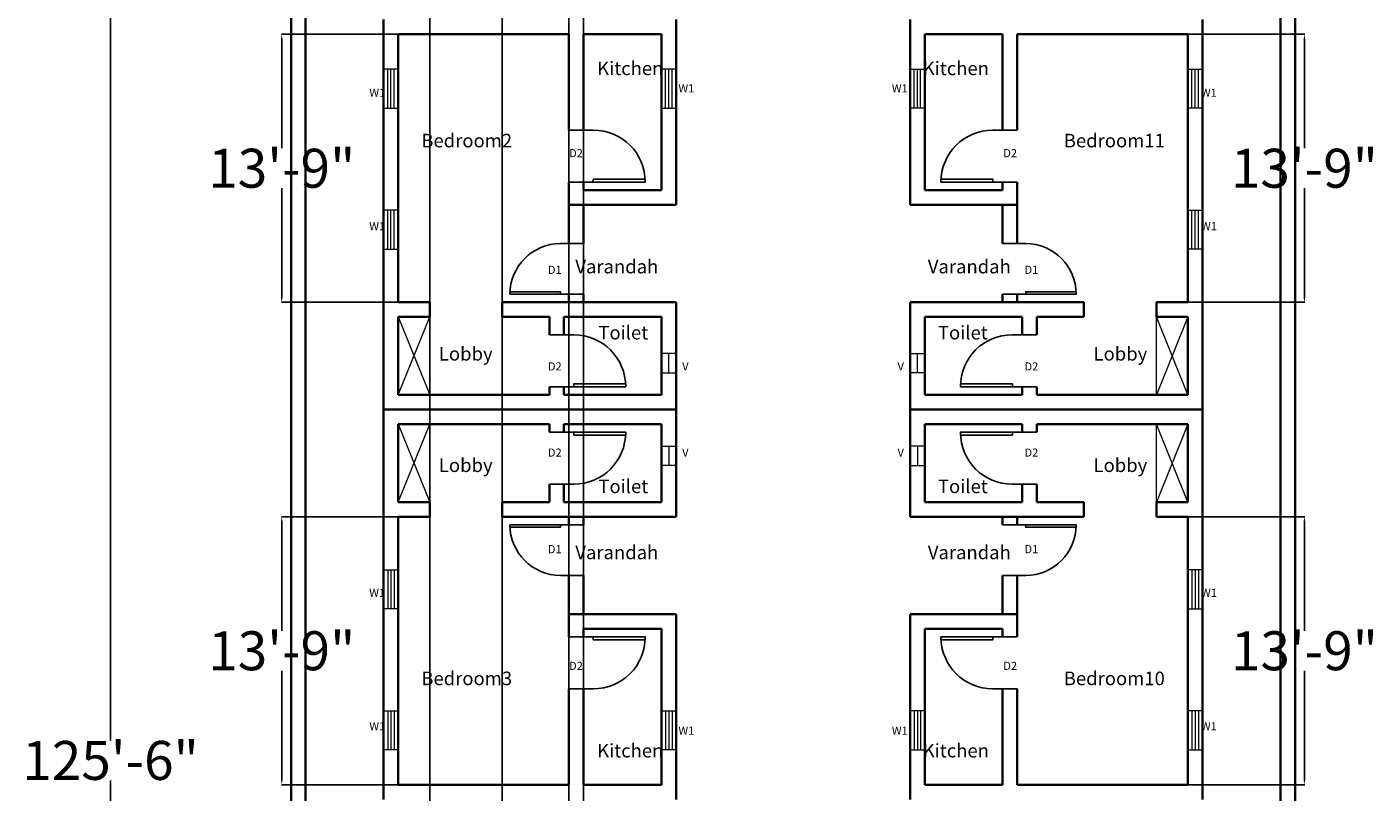
# Model space of a CAD drawing. Units: inches. Extents: x -205 to 674, y 63 to 1798.
# Tile 2 of 4: x -205 to 624, y 888 to 1359. Entities that reach past the tile are written whole.
import ezdxf

# ---------------------------------------------------------------- set-up
doc = ezdxf.new("R2010")
doc.units = ezdxf.units.IN
doc.header["$MEASUREMENT"] = 0
doc.layers.get('0').update_dxf_attribs({"color": 70})
for name, color, linetype, lineweight in [('A-ANNO-DIMS', 240, 'Continuous', 18), ('A-ANNO-TEXT', 240, 'Continuous', 18), ('A-AREA-IDEN', 240, 'Continuous', 18), ('A-WALL', 70, 'Continuous', 35), ('A-WALL-SITE', 70, 'Continuous', 35), ('door1', 20, 'Continuous', 25), ('door2', 160, 'Continuous', 25), ('lobby', 241, 'Continuous', 18), ('ventilator1', 210, 'Continuous', 18), ('window1', 50, 'Continuous', 18)]:
    doc.layers.add(name, color=color, linetype=linetype, lineweight=lineweight)
doc.styles.get("Standard").update_dxf_attribs({"font": 'arial.ttf'})
doc.dimstyles.get("Standard").update_dxf_attribs({"dimtxt": 5, "dimasz": 3, "dimexe": 0.18, "dimexo": 0.0625, "dimgap": 0.09, "dimtad": 0, "dimtih": 1, "dimtoh": 1, "dimdec": 0, "dimzin": 0, "dimdsep": 46, "dimlunit": 3, "dimtxsty": 'Standard', "dimcen": 0.09, "dimadec": 0, "dimazin": 0, "dimtfac": 1, "dimtdec": 0, "dimtofl": 0, "dimtmove": 0, "dimatfit": 3, "dimfxl": 1, "dimtolj": 1, "dimtzin": 0, "dimarcsym": 0})

# ---------------------------------------------------------------- blocks, each defined once
blk = doc.blocks.new('*D6')
at = {"layer": 'A-ANNO-DIMS', "color": 0, "lineweight": -2, "transparency": 16777216}
for p, q in [((23.48, 1354.3), (-48.36, 1354.3)), ((-48.18, 1351.3), (-48.18, 1284.15)), ((-48.18, 1192.3), (-48.18, 1259.45)), ((23.48, 1189.3), (-48.36, 1189.3))]:
    blk.add_line(p, q, dxfattribs=at)
at = {"layer": 'A-ANNO-DIMS', "color": 0, "transparency": 16777216}
for points in [[(-48.68, 1351.3), (-47.68, 1351.3), (-48.18, 1354.3)], [(-48.68, 1192.3), (-47.68, 1192.3), (-48.18, 1189.3)]]:
    blk.add_solid(points, dxfattribs=at)
at = {"layer": 'Defpoints', "color": 0, "transparency": 16777216}
for p in [(-48.18, 1354.3), (23.54, 1354.3), (23.54, 1189.3)]:
    blk.add_point(p, dxfattribs=at)
at = {"layer": 'A-ANNO-DIMS', "color": 0, "transparency": 16777216, "insert": (-48.18, 1271.8), "char_height": 5, "attachment_point": 5}
blk.add_mtext('\\A1;{\\H4.8x;13\'-9"}', dxfattribs=at)
blk = doc.blocks.new('*U4')
for p, q in [((0, 0), (0, -6)), ((36, 0), (36, -6))]:
    blk.add_line(p, q)
blk.add_lwpolyline([(0, 0), (0, 36), (1.75, 36), (1.75, 0)], close=True)
blk.add_arc((0, 0), 36, 0, 90)
blk = doc.blocks.new('*U5')
for p, q in [((0, 0), (0, -6)), ((32, 0), (32, -6))]:
    blk.add_line(p, q)
blk.add_lwpolyline([(0, 0), (0, 32), (1.75, 32), (1.75, 0)], close=True)
blk.add_arc((0, 0), 32, 0, 90)
blk = doc.blocks.new('*D7')
at = {"layer": 'A-ANNO-DIMS', "color": 0, "lineweight": -2, "transparency": 16777216}
for p, q in [((23.48, 1057.3), (-48.36, 1057.3)), ((-48.18, 1054.3), (-48.18, 987.15)), ((-48.18, 895.3), (-48.18, 962.45)), ((23.48, 892.3), (-48.36, 892.3))]:
    blk.add_line(p, q, dxfattribs=at)
at = {"layer": 'A-ANNO-DIMS', "color": 0, "transparency": 16777216}
for points in [[(-48.68, 1054.3), (-47.68, 1054.3), (-48.18, 1057.3)], [(-48.68, 895.3), (-47.68, 895.3), (-48.18, 892.3)]]:
    blk.add_solid(points, dxfattribs=at)
at = {"layer": 'Defpoints', "color": 0, "transparency": 16777216}
for p in [(23.54, 1057.3), (-48.18, 892.3), (23.54, 892.3)]:
    blk.add_point(p, dxfattribs=at)
at = {"layer": 'A-ANNO-DIMS', "color": 0, "transparency": 16777216, "insert": (-48.18, 974.8), "char_height": 5, "attachment_point": 5}
blk.add_mtext('\\A1;{\\H4.8x;13\'-9"}', dxfattribs=at)
blk = doc.blocks.new('*D11')
at = {"layer": 'A-ANNO-DIMS', "color": 0, "lineweight": -2, "transparency": 16777216}
for p, q in [((509.6, 1354.3), (581.44, 1354.3)), ((581.26, 1351.3), (581.26, 1284.15)), ((581.26, 1192.3), (581.26, 1259.45)), ((509.6, 1189.3), (581.44, 1189.3))]:
    blk.add_line(p, q, dxfattribs=at)
at = {"layer": 'A-ANNO-DIMS', "color": 0, "transparency": 16777216}
for points in [[(580.76, 1351.3), (581.76, 1351.3), (581.26, 1354.3)], [(580.76, 1192.3), (581.76, 1192.3), (581.26, 1189.3)]]:
    blk.add_solid(points, dxfattribs=at)
at = {"layer": 'Defpoints', "color": 0, "transparency": 16777216}
for p in [(509.54, 1354.3), (581.26, 1354.3), (509.54, 1189.3)]:
    blk.add_point(p, dxfattribs=at)
at = {"layer": 'A-ANNO-DIMS', "color": 0, "transparency": 16777216, "insert": (581.26, 1271.8), "char_height": 5, "attachment_point": 5}
blk.add_mtext('\\A1;{\\H4.8x;13\'-9"}', dxfattribs=at)
blk = doc.blocks.new('*D14')
at = {"layer": 'A-ANNO-DIMS', "color": 0, "lineweight": -2, "transparency": 16777216}
for p, q in [((509.6, 1057.3), (581.44, 1057.3)), ((581.26, 1054.3), (581.26, 987.15)), ((581.26, 895.3), (581.26, 962.45)), ((509.6, 892.3), (581.44, 892.3))]:
    blk.add_line(p, q, dxfattribs=at)
at = {"layer": 'A-ANNO-DIMS', "color": 0, "transparency": 16777216}
for points in [[(580.76, 1054.3), (581.76, 1054.3), (581.26, 1057.3)], [(580.76, 895.3), (581.76, 895.3), (581.26, 892.3)]]:
    blk.add_solid(points, dxfattribs=at)
at = {"layer": 'Defpoints', "color": 0, "transparency": 16777216}
for p in [(509.54, 1057.3), (509.54, 892.3), (581.26, 892.3)]:
    blk.add_point(p, dxfattribs=at)
at = {"layer": 'A-ANNO-DIMS', "color": 0, "transparency": 16777216, "insert": (581.26, 974.8), "char_height": 5, "attachment_point": 5}
blk.add_mtext('\\A1;{\\H4.8x;13\'-9"}', dxfattribs=at)
blk = doc.blocks.new('*D18')
at = {"layer": 'A-ANNO-DIMS', "color": 0, "lineweight": -2, "transparency": 16777216}
for p, q in [((-42.52, 1660.3), (-153.74, 1660.3)), ((-153.56, 1657.3), (-153.56, 919.64)), ((-153.56, 157.3), (-153.56, 894.96)), ((-42.52, 154.3), (-153.74, 154.3))]:
    blk.add_line(p, q, dxfattribs=at)
at = {"layer": 'A-ANNO-DIMS', "color": 0, "transparency": 16777216}
for points in [[(-154.06, 1657.3), (-153.06, 1657.3), (-153.56, 1660.3)], [(-154.06, 157.3), (-153.06, 157.3), (-153.56, 154.3)]]:
    blk.add_solid(points, dxfattribs=at)
at = {"layer": 'Defpoints', "color": 0, "transparency": 16777216}
for p in [(-42.46, 1660.3), (-153.56, 154.3), (-42.46, 154.3)]:
    blk.add_point(p, dxfattribs=at)
at = {"layer": 'A-ANNO-DIMS', "color": 0, "transparency": 16777216, "insert": (-153.56, 907.3), "char_height": 5, "attachment_point": 5}
blk.add_mtext('\\A1;{\\H4.8x;125\'-6"}', dxfattribs=at)
blk = doc.blocks.new('WIN-W1-24IN')
for p, q in [((2.5, 24), (2.5, 0)), ((4.5, 24), (4.5, 0)), ((6.5, 24), (6.5, 0))]:
    blk.add_line(p, q)
blk.add_lwpolyline([(0, 24), (9, 24), (9, 0), (0, 0)], close=True)
blk = doc.blocks.new('VENT-V-12IN')
blk.add_line((4.5, 12), (4.5, 0))
blk.add_lwpolyline([(9, 0), (0, 0), (0, 12), (9, 12)], close=True)
blk = doc.blocks.new('LOBBY-RECESS')
for p, q in [((0, 48), (19.36, 0)), ((0, 0), (19.36, 48)), ((19.36, 48), (19.36, 0))]:
    blk.add_line(p, q)
blk = doc.blocks.new('*D40')
at = {"layer": 'A-ANNO-DIMS', "color": 0, "lineweight": -2, "transparency": 16777216}
for p, q in [((128.54, 1372.24), (128.54, 69.92)), ((137.54, 1372.24), (137.54, 69.92)), ((131.54, 70.1), (134.54, 70.1)), ((137.54, 70.1), (140.54, 70.1))]:
    blk.add_line(p, q, dxfattribs=at)
at = {"layer": 'A-ANNO-DIMS', "color": 0, "transparency": 16777216}
for points in [[(131.54, 70.6), (131.54, 69.6), (128.54, 70.1)], [(134.54, 70.6), (134.54, 69.6), (137.54, 70.1)]]:
    blk.add_solid(points, dxfattribs=at)
at = {"layer": 'Defpoints', "color": 0, "transparency": 16777216}
for p in [(128.54, 1372.3), (137.54, 1372.3), (137.54, 70.1)]:
    blk.add_point(p, dxfattribs=at)
at = {"layer": 'A-ANNO-DIMS', "color": 0, "transparency": 16777216, "insert": (147.28, 70.1), "char_height": 5, "attachment_point": 5}
blk.add_mtext('\\A1;0\'-9"', dxfattribs=at)
blk = doc.blocks.new('*D47')
at = {"layer": 'A-ANNO-DIMS', "color": 0, "lineweight": -2, "transparency": 16777216}
for p, q in [((42.9, 1546.24), (42.9, 69.92)), ((87.49, 1546.24), (87.49, 69.92)), ((45.9, 70.1), (52.64, 70.1)), ((84.49, 70.1), (77.76, 70.1))]:
    blk.add_line(p, q, dxfattribs=at)
at = {"layer": 'A-ANNO-DIMS', "color": 0, "transparency": 16777216}
for points in [[(45.9, 70.6), (45.9, 69.6), (42.9, 70.1)], [(84.49, 70.6), (84.49, 69.6), (87.49, 70.1)]]:
    blk.add_solid(points, dxfattribs=at)
at = {"layer": 'Defpoints', "color": 0, "transparency": 16777216}
for p in [(42.9, 1546.3), (87.49, 1546.3), (87.49, 70.1)]:
    blk.add_point(p, dxfattribs=at)
at = {"layer": 'A-ANNO-DIMS', "color": 0, "transparency": 16777216, "insert": (65.2, 70.1), "char_height": 5, "attachment_point": 5}
blk.add_mtext('\\A1;3\'-8 1/2"', dxfattribs=at)

msp = doc.modelspace()

# ---------------------------------------------------------------- linework, layer by layer
at = {"layer": 'A-WALL'}
for p, q in [((14.54, 1363.3), (14.54, 1123.3)), ((194.54, 1249.3), (194.54, 1363.3)), ((338.54, 1249.3), (338.54, 1363.3)), ((518.54, 1363.3), (518.54, 1123.3)), ((128.54, 1354.3), (23.54, 1354.3)), ((23.54, 1354.3), (23.54, 1189.3)), ((128.54, 1295.3), (128.54, 1354.3)), ((137.54, 1295.3), (137.54, 1354.3)), ((185.54, 1354.3), (137.54, 1354.3)), ((137.54, 1295.3), (137.54, 1354.3)), ((185.54, 1258.3), (185.54, 1354.3)), ((347.54, 1258.3), (347.54, 1354.3)), ((347.54, 1354.3), (395.54, 1354.3)), ((395.54, 1295.3), (395.54, 1354.3)), ((395.54, 1295.3), (395.54, 1354.3)), ((404.54, 1295.3), (404.54, 1354.3)), ((404.54, 1354.3), (509.54, 1354.3)), ((509.54, 1354.3), (509.54, 1189.3)), ((128.54, 1225.41), (128.54, 1263.3)), ((128.54, 1263.3), (128.54, 1258.3)), ((137.54, 1258.3), (137.54, 1263.3)), ((137.54, 1258.3), (137.54, 1263.3)), ((395.54, 1258.3), (395.54, 1263.3)), ((395.54, 1258.3), (395.54, 1263.3)), ((404.54, 1225.41), (404.54, 1263.3)), ((404.54, 1263.3), (404.54, 1258.3)), ((185.54, 1258.3), (137.54, 1258.3)), ((347.54, 1258.3), (395.54, 1258.3)), ((194.54, 1249.3), (128.54, 1249.3)), ((137.54, 1225.41), (137.54, 1249.3)), ((338.54, 1249.3), (404.54, 1249.3)), ((395.54, 1225.41), (395.54, 1249.3)), ((128.54, 1189.3), (128.54, 1194.3)), ((137.54, 1189.3), (137.54, 1194.3)), ((137.55, 1189.3), (137.55, 1194.2)), ((395.54, 1189.3), (395.54, 1194.3)), ((395.54, 1189.3), (395.54, 1194.2)), ((404.54, 1189.3), (404.54, 1194.3)), ((23.54, 1189.3), (42.9, 1189.3)), ((42.9, 1180.3), (42.9, 1189.3)), ((42.9, 1189.3), (42.9, 1189.3)), ((87.49, 1189.3), (194.54, 1189.3)), ((87.49, 1180.3), (87.49, 1189.3)), ((87.49, 1189.3), (87.49, 1189.3)), ((194.54, 1123.3), (194.54, 1189.3)), ((338.54, 1123.3), (338.54, 1189.3)), ((445.59, 1189.3), (338.54, 1189.3)), ((445.59, 1180.3), (445.59, 1189.3)), ((445.59, 1189.3), (445.59, 1189.3)), ((509.54, 1189.3), (490.18, 1189.3)), ((490.18, 1180.3), (490.18, 1189.3)), ((490.18, 1189.3), (490.18, 1189.3)), ((23.54, 1180.3), (42.9, 1180.3)), ((23.54, 1180.3), (23.54, 1132.3)), ((87.49, 1180.3), (116.54, 1180.3)), ((116.54, 1169.3), (116.54, 1180.3)), ((125.54, 1180.3), (185.54, 1180.3)), ((125.54, 1169.3), (125.54, 1180.3)), ((185.54, 1132.3), (185.54, 1180.3)), ((407.54, 1180.3), (347.54, 1180.3)), ((347.54, 1132.3), (347.54, 1180.3)), ((407.54, 1169.3), (407.54, 1180.3)), ((445.59, 1180.3), (416.54, 1180.3)), ((416.54, 1169.3), (416.54, 1180.3)), ((509.54, 1180.3), (490.18, 1180.3)), ((509.54, 1180.3), (509.54, 1132.3)), ((116.54, 1132.3), (116.54, 1137.3)), ((116.54, 1137.3), (116.54, 1132.3)), ((125.54, 1132.3), (125.54, 1137.3)), ((125.54, 1132.3), (125.54, 1137.3)), ((407.54, 1132.3), (407.54, 1137.3)), ((407.54, 1132.3), (407.54, 1137.3)), ((416.54, 1132.3), (416.54, 1137.3)), ((416.54, 1137.3), (416.54, 1132.3)), ((23.54, 1132.3), (116.54, 1132.3)), ((125.54, 1132.3), (185.54, 1132.3)), ((407.54, 1132.3), (347.54, 1132.3)), ((509.54, 1132.3), (416.54, 1132.3)), ((14.54, 1123.3), (194.54, 1123.3)), ((14.54, 1123.3), (194.54, 1123.3)), ((14.54, 883.3), (14.54, 1123.3)), ((194.54, 1123.3), (194.54, 1057.3)), ((518.54, 1123.3), (338.54, 1123.3)), ((518.54, 1123.3), (338.54, 1123.3)), ((338.54, 1123.3), (338.54, 1057.3)), ((518.54, 883.3), (518.54, 1123.3)), ((23.54, 1114.3), (116.54, 1114.3)), ((23.54, 1066.3), (23.54, 1114.3)), ((116.54, 1114.3), (116.54, 1109.3)), ((116.54, 1109.3), (116.54, 1114.3)), ((125.54, 1114.3), (185.54, 1114.3)), ((125.54, 1114.3), (125.54, 1109.3)), ((125.54, 1114.3), (125.54, 1109.3)), ((185.54, 1114.3), (185.54, 1066.3)), ((407.54, 1114.3), (347.54, 1114.3)), ((347.54, 1114.3), (347.54, 1066.3)), ((407.54, 1114.3), (407.54, 1109.3)), ((407.54, 1114.3), (407.54, 1109.3)), ((509.54, 1114.3), (416.54, 1114.3)), ((416.54, 1114.3), (416.54, 1109.3)), ((416.54, 1109.3), (416.54, 1114.3)), ((509.54, 1066.3), (509.54, 1114.3)), ((116.54, 1077.3), (116.54, 1066.3)), ((125.54, 1077.3), (125.54, 1066.3)), ((407.54, 1077.3), (407.54, 1066.3)), ((416.54, 1077.3), (416.54, 1066.3)), ((23.54, 1066.3), (42.9, 1066.3)), ((42.9, 1066.3), (42.9, 1057.3)), ((87.49, 1066.3), (116.54, 1066.3)), ((87.49, 1066.3), (87.49, 1057.3)), ((125.54, 1066.3), (185.54, 1066.3)), ((407.54, 1066.3), (347.54, 1066.3)), ((445.59, 1066.3), (416.54, 1066.3)), ((445.59, 1066.3), (445.59, 1057.3)), ((509.54, 1066.3), (490.18, 1066.3)), ((490.18, 1066.3), (490.18, 1057.3)), ((23.54, 1057.3), (42.9, 1057.3)), ((23.54, 892.3), (23.54, 1057.3)), ((42.9, 1057.3), (42.9, 1057.3)), ((87.49, 1057.3), (194.54, 1057.3)), ((87.49, 1057.3), (87.49, 1057.3)), ((128.54, 1057.3), (128.54, 1052.3)), ((137.54, 1057.3), (137.54, 1052.3)), ((137.55, 1057.29), (137.55, 1052.4)), ((445.59, 1057.3), (338.54, 1057.3)), ((395.54, 1057.3), (395.54, 1052.3)), ((395.54, 1057.29), (395.54, 1052.4)), ((404.54, 1057.3), (404.54, 1052.3)), ((445.59, 1057.3), (445.59, 1057.3)), ((509.54, 1057.3), (490.18, 1057.3)), ((490.18, 1057.3), (490.18, 1057.3)), ((509.54, 892.3), (509.54, 1057.3)), ((128.54, 1021.19), (128.54, 983.3)), ((137.54, 1021.19), (137.54, 997.3)), ((395.54, 1021.19), (395.54, 997.3)), ((404.54, 1021.19), (404.54, 983.3)), ((194.54, 997.3), (128.54, 997.3)), ((194.54, 997.3), (194.54, 883.3)), ((338.54, 997.3), (338.54, 883.3)), ((338.54, 997.3), (404.54, 997.3)), ((128.54, 983.3), (128.54, 988.3)), ((137.54, 988.3), (137.54, 983.3)), ((185.54, 988.3), (137.54, 988.3)), ((137.54, 988.3), (137.54, 983.3)), ((185.54, 988.3), (185.54, 892.3)), ((347.54, 988.3), (347.54, 892.3)), ((347.54, 988.3), (395.54, 988.3)), ((395.54, 988.3), (395.54, 983.3)), ((395.54, 988.3), (395.54, 983.3)), ((404.54, 983.3), (404.54, 988.3)), ((128.54, 951.3), (128.54, 892.3)), ((137.54, 951.3), (137.54, 892.3)), ((137.54, 951.3), (137.54, 892.3)), ((395.54, 951.3), (395.54, 892.3)), ((395.54, 951.3), (395.54, 892.3)), ((404.54, 951.3), (404.54, 892.3)), ((128.54, 892.3), (23.54, 892.3)), ((185.54, 892.3), (137.54, 892.3)), ((347.54, 892.3), (395.54, 892.3)), ((404.54, 892.3), (509.54, 892.3))]:
    msp.add_line(p, q, dxfattribs=at)
at = {"layer": 'A-WALL-SITE'}
for points in [[(575.54, 154.3), (575.54, 1660.3), (266.54, 1660.3), (-42.46, 1660.3), (-42.46, 154.3), (266.54, 154.3)], [(566.54, 163.3), (566.54, 1651.3), (266.54, 1651.3), (-33.46, 1651.3), (-33.46, 163.3), (266.54, 163.3)]]:
    msp.add_lwpolyline(points, close=True, dxfattribs=at)
at = {"layer": 'door1'}
for p, q in [((128.54, 1225.41), (137.54, 1225.41)), ((404.54, 1225.41), (395.54, 1225.41)), ((128.54, 1194.3), (137.54, 1194.3)), ((404.54, 1194.3), (395.54, 1194.3)), ((128.54, 1052.3), (137.54, 1052.3)), ((404.54, 1052.3), (395.54, 1052.3)), ((128.54, 1021.19), (137.54, 1021.19)), ((404.54, 1021.19), (395.54, 1021.19))]:
    msp.add_line(p, q, dxfattribs=at)
at = {"layer": 'door2'}
for p, q in [((137.54, 1295.3), (128.54, 1295.3)), ((395.54, 1295.3), (404.54, 1295.3)), ((128.54, 1263.3), (137.54, 1263.3)), ((404.54, 1263.3), (395.54, 1263.3)), ((125.54, 1169.3), (116.54, 1169.3)), ((407.54, 1169.3), (416.54, 1169.3)), ((116.54, 1137.3), (125.54, 1137.3)), ((416.54, 1137.3), (407.54, 1137.3)), ((116.54, 1109.3), (125.54, 1109.3)), ((416.54, 1109.3), (407.54, 1109.3)), ((125.54, 1077.3), (116.54, 1077.3)), ((407.54, 1077.3), (416.54, 1077.3)), ((128.54, 983.3), (137.54, 983.3)), ((404.54, 983.3), (395.54, 983.3)), ((137.54, 951.3), (128.54, 951.3)), ((395.54, 951.3), (404.54, 951.3))]:
    msp.add_line(p, q, dxfattribs=at)

# ---------------------------------------------------------------- block references
at = {"layer": 'door1', "yscale": 0.8640557789234337, "zscale": 0.8640557789234337}
for p, xscale, rotation in [((123.36, 1194.3), 0.8640557789234337, 90.00000000000003), ((409.73, 1194.3), -0.8640557789234337, 270), ((123.36, 1052.3), -0.8640557789234337, 90), ((409.73, 1052.3), 0.8640557789234337, 270)]:
    msp.add_blockref('*U4', p, dxfattribs=dict(at, xscale=xscale, rotation=rotation))
at = {"layer": 'door2', "xscale": -1}
for p, rotation in [((143.54, 1263.3), 270), ((131.54, 1137.3), 270), ((401.54, 1109.3), 90), ((389.54, 983.3), 90)]:
    msp.add_blockref('*U5', p, dxfattribs=dict(at, rotation=rotation))
at = {"layer": 'door2'}
for p, rotation in [((389.54, 1263.3), 90.00000000000003), ((401.54, 1137.3), 90.00000000000003), ((131.54, 1109.3), 270), ((143.54, 983.3), 270)]:
    msp.add_blockref('*U5', p, dxfattribs=dict(at, rotation=rotation))
at = {"layer": 'lobby'}
for p in [(23.54, 1132.3), (23.54, 1066.3)]:
    msp.add_blockref('LOBBY-RECESS', p, dxfattribs=at)
at = {"layer": 'lobby', "rotation": 180}
for p in [(509.54, 1180.3), (509.54, 1114.3)]:
    msp.add_blockref('LOBBY-RECESS', p, dxfattribs=at)
at = {"layer": 'ventilator1', "extrusion": (0, 0, -1), "zscale": -1, "rotation": 180}
msp.add_blockref('VENT-V-12IN', (-185.54, 1157.85), dxfattribs=at)
at = {"layer": 'ventilator1', "rotation": 180}
msp.add_blockref('VENT-V-12IN', (347.54, 1157.85), dxfattribs=at)
at = {"layer": 'ventilator1'}
msp.add_blockref('VENT-V-12IN', (185.54, 1088.75), dxfattribs=at)
at = {"layer": 'ventilator1', "extrusion": (0, 0, -1), "zscale": -1}
msp.add_blockref('VENT-V-12IN', (-347.54, 1088.75), dxfattribs=at)
at = {"layer": 'window1', "extrusion": (0, 0, -1), "zscale": -1, "rotation": 180}
for p in [(-14.54, 1332.79), (-185.54, 1332.79), (-14.54, 1246.03)]:
    msp.add_blockref('WIN-W1-24IN', p, dxfattribs=at)
at = {"layer": 'window1', "rotation": 180}
for p in [(347.54, 1332.79), (518.54, 1332.79), (518.54, 1246.03)]:
    msp.add_blockref('WIN-W1-24IN', p, dxfattribs=at)
at = {"layer": 'window1'}
for p in [(14.54, 1000.57), (14.54, 913.81), (185.54, 913.81)]:
    msp.add_blockref('WIN-W1-24IN', p, dxfattribs=at)
at = {"layer": 'window1', "extrusion": (0, 0, -1), "zscale": -1}
for p in [(-518.54, 1000.57), (-347.54, 913.81), (-518.54, 913.81)]:
    msp.add_blockref('WIN-W1-24IN', p, dxfattribs=at)

# ---------------------------------------------------------------- texts
at = {"layer": 'A-ANNO-TEXT', "char_height": 5}
for s, insert, attachment_point in [('W1', (5.74, 1315.77), 7), ('W1', (195.97, 1318.49), 7), ('W1', (337.12, 1318.49), 9), ('W1', (527.34, 1315.77), 9), ('D2', (128.68, 1278.61), 7), ('D2', (404.41, 1278.61), 9), ('W1', (5.68, 1233.64), 7), ('W1', (527.4, 1233.64), 9), ('D1', (115.64, 1206.76), 7), ('D1', (417.45, 1206.76), 9), ('D2', (115.64, 1147.31), 7), ('V', (198.3, 1147.31), 7), ('V', (334.78, 1147.31), 9), ('D2', (417.45, 1147.31), 9), ('D2', (115.64, 1099.29), 1), ('V', (198.3, 1099.29), 1), ('V', (334.78, 1099.29), 3), ('D2', (417.45, 1099.29), 3), ('D1', (115.64, 1039.84), 1), ('D1', (417.45, 1039.84), 3), ('W1', (5.68, 1012.96), 1), ('W1', (527.4, 1012.96), 3), ('D2', (128.68, 967.99), 1), ('D2', (404.41, 967.99), 3), ('W1', (5.74, 930.83), 1), ('W1', (195.97, 928.11), 1), ('W1', (337.12, 928.11), 3), ('W1', (527.34, 930.83), 3)]:
    msp.add_mtext_dynamic_manual_height_columns(s, width=13.5017, gutter_width=1, heights=[0], dxfattribs=dict(at, insert=insert, attachment_point=attachment_point))
at = {"layer": 'A-AREA-IDEN', "char_height": 8.34}
for s, insert, attachment_point in [('Kitchen', (145.99, 1329.12), 7), ('Kitchen', (387.1, 1329.12), 9), ('Bedroom2', (37.73, 1284.65), 7), ('Bedroom11', (495.36, 1284.65), 9), ('Varandah', (132.52, 1207.11), 7), ('Varandah', (400.56, 1207.11), 9), ('Toilet', (146.71, 1166.44), 7), ('Toilet', (386.37, 1166.44), 9), ('Lobby', (48.54, 1153.43), 7), ('Lobby', (484.55, 1153.43), 9), ('Lobby', (48.54, 1093.17), 1), ('Lobby', (484.55, 1093.17), 3), ('Toilet', (146.71, 1080.16), 1), ('Toilet', (386.37, 1080.16), 3), ('Varandah', (132.52, 1039.49), 1), ('Varandah', (400.56, 1039.49), 3), ('Bedroom3', (37.73, 961.95), 1), ('Bedroom10', (495.36, 961.95), 3), ('Kitchen', (145.99, 917.47), 1), ('Kitchen', (387.1, 917.47), 3)]:
    msp.add_mtext_dynamic_manual_height_columns(s, width=37.3149, gutter_width=1.67, heights=[0], dxfattribs=dict(at, insert=insert, attachment_point=attachment_point))

# ---------------------------------------------------------------- dimensions: what is measured, and where the dimension line sits
at = {"layer": 'A-ANNO-DIMS'}
for base, p1, p2, angle, picture, middle in [((-153.56, 154.3), (-42.46, 1660.3), (-42.46, 154.3), 90, '*D18', (-153.56, 907.3)), ((-48.18, 1354.3), (23.54, 1189.3), (23.54, 1354.3), 270, '*D6', (-48.18, 1271.8)), ((581.26, 1354.3), (509.54, 1189.3), (509.54, 1354.3), 270, '*D11', (581.26, 1271.8)), ((-48.18, 892.3), (23.54, 1057.3), (23.54, 892.3), 90, '*D7', (-48.18, 974.8)), ((581.26, 892.3), (509.54, 1057.3), (509.54, 892.3), 90, '*D14', (581.26, 974.8))]:
    dim = msp.add_linear_dim(base=base, p1=p1, p2=p2, angle=angle, text='{\\H4.8x;<>}', dimstyle='Standard', override={"dimclrd": 0, "dimclre": 0, "dimclrt": 0}, dxfattribs=at)
    dim.commit()
    dim.dimension.update_dxf_attribs({"geometry": picture, "text_midpoint": middle})
for base, p1, p2, picture, middle in [((87.49, 70.1), (42.9, 1546.3), (87.49, 1546.3), '*D47', (65.2, 70.1)), ((137.54, 70.1), (128.54, 1372.3), (137.54, 1372.3), '*D40', (147.28, 70.1))]:
    dim = msp.add_linear_dim(base=base, p1=p1, p2=p2, dimstyle='Standard', override={"dimdec": 1, "dimlfac": 1, "dimrnd": 0, "dimzin": 1, "dimdsep": 46, "dimlunit": 4, "dimfrac": 2}, dxfattribs=at)
    dim.commit()
    dim.dimension.update_dxf_attribs({"geometry": picture, "text_midpoint": middle})

doc.saveas('drawing.dxf')
